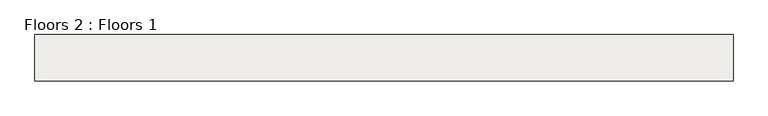
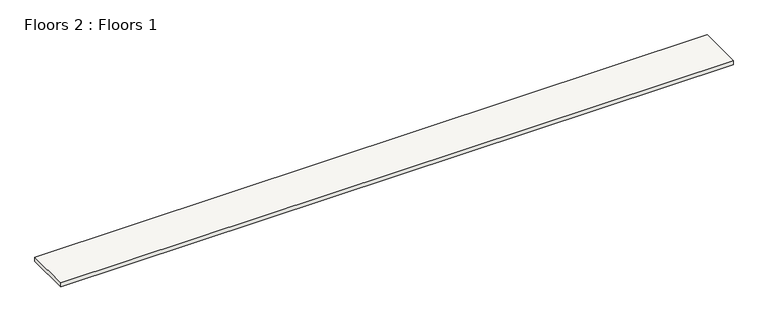
"""IFC4 building model written with IfcOpenShell, lengths in millimetres: slab geometry, Floors 2 : Floors 1."""

from ifc_helpers import new_model, si_unit, frame, origin, place, context, project, spatial, polyline, outline, extrude, source, transform, mapped, element, save


def floors_2_floors_1_5c930e2b(model_context):
    return source(origin(), model_context, "Body", "SweptSolid", [
        extrude(outline(polyline([(41445.3647012, -963.9627409), (14013.3647012, -963.9627409), (14013.3647012, 864.8372591), (41445.3647012, 864.8372591), (41445.3647012, -963.9627409)])), frame((0.0, 0.0, -304.8), z_axis=(0.0, 0.0, 1.0), x_axis=(1.0, 0.0, 0.0)), (0.0, 0.0, 1.0), 172.7176062),
    ])


if __name__ == "__main__":
    model = new_model("IFC4")
    model_context = context("Model", 3, world=origin())
    ifc_project = project(units=[si_unit("LENGTHUNIT", "METRE", prefix="MILLI")], contexts=[model_context])
    site = spatial("IfcSite", under=ifc_project)
    building = spatial("IfcBuilding", under=site)
    placement = place(None, origin())
    floors_2_floors_1_shape = floors_2_floors_1_5c930e2b(model_context)
    element("IfcSlab", 1, ObjectType="Floors 2 : Floors 1", at=placement, inside=building, context=model_context, shape_type="MappedRepresentation", body=[
        mapped(floors_2_floors_1_shape, transform((0.0, 0.0, 0.0), x_axis=(1.0, 0.0, 0.0), y_axis=(0.0, 1.0, 0.0), z_axis=(0.0, 0.0, 1.0))),
    ])
    save(model, "model.ifc")

# Revit data of these elements
# Element 1 (IfcSlab, "Floors 2 : Floors 1")
#   Materials on its faces: "Concrete, Cast-in-Place gray"
# Materials
#   "Concrete, Cast-in-Place gray": class "Concrete", colour RGB 192 192 192, transparency 0, Description = "Cast-in-place concrete", Cost = 0
